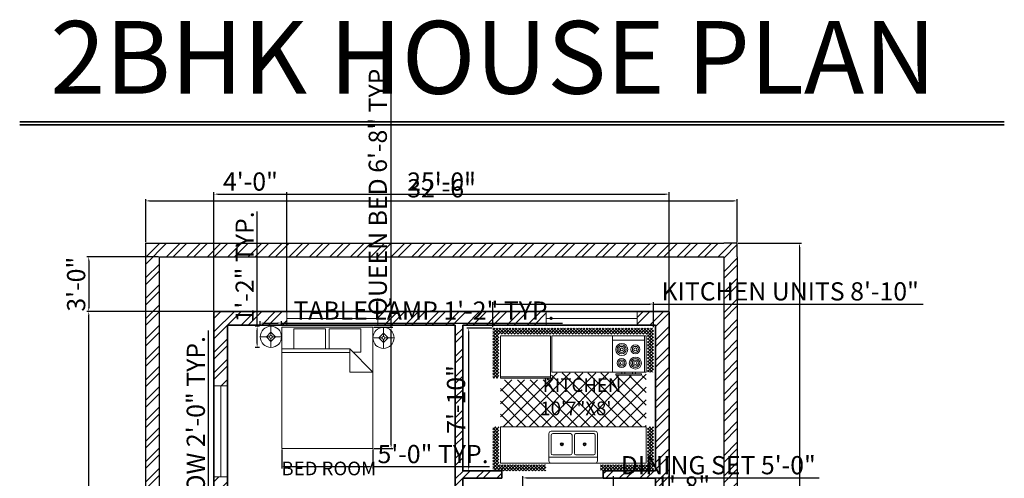
# Model space of a CAD drawing. Units: inches. Extents: x 2588 to 3237, y 2402 to 3178.
# Tile 4 of 4: x 2588 to 3237, y 2876 to 3178. Entities that reach past the tile are written whole.
import ezdxf

# ---------------------------------------------------------------- set-up
doc = ezdxf.new("R2010")
doc.units = ezdxf.units.IN
for name, color, linetype, lineweight in [('A-ANNO-DIMS', 2, 'Continuous', 18), ('A-ANNO-TITL', 7, 'Continuous', 35), ('A-AREA-IDEN', 7, 'Continuous', 25), ('A-FLOR-FIXT', 9, 'Continuous', 18), ('A-FURN', 8, 'Continuous', 18), ('A-GLAZ', 4, 'Continuous', 18), ('A-WALL-PATT', 252, 'Continuous', 13), ('L-WALL', 7, 'Continuous', 30), ('L-WALL-PATT', 252, 'Continuous', 13), ('wall', 210, 'Continuous', 35)]:
    doc.layers.add(name, color=color, linetype=linetype, lineweight=lineweight)
doc.styles.get("Standard").update_dxf_attribs({"font": 'arial.ttf'})
doc.dimstyles.new('ISO-25', dxfattribs={"dimtxt": 12, "dimasz": 2.5, "dimexe": 1.25, "dimexo": 0.625, "dimtad": 1, "dimdec": 1, "dimlunit": 4, "dimtxsty": 'Standard', "dimcen": 2.5, "dimadec": 0, "dimazin": 0, "dimtfac": 1, "dimtdec": 1, "dimtmove": 0, "dimatfit": 3, "dimfxl": 1, "dimarcsym": 0})

# ---------------------------------------------------------------- blocks, each defined once
blk = doc.blocks.new('Kitchen Layout - 7 x 8 ft')
for p, q in [((-5, 81.32), (2.68, 89)), ((-5, 83.44), (0.56, 89)), ((-5, 85.56), (-1.56, 89)), ((-5, 87.68), (-3.68, 89)), ((-1, 84.97), (-5, 88.97)), ((-1, 82.85), (-5, 86.85)), ((-1, 80.73), (-5, 84.73)), ((1.09, 85), (-2.91, 89)), ((3.21, 85), (-0.79, 89)), ((0.81, 85), (4.81, 89)), ((5.34, 85), (1.34, 89)), ((2.93, 85), (6.93, 89)), ((7.46, 85), (3.46, 89)), ((5.05, 85), (9.05, 89)), ((9.58, 85), (5.58, 89)), ((7.17, 85), (11.17, 89)), ((11.7, 85), (7.7, 89)), ((9.29, 85), (13.29, 89)), ((13.82, 85), (9.82, 89)), ((11.41, 85), (15.41, 89)), ((15.94, 85), (11.94, 89)), ((13.53, 85), (17.53, 89)), ((18.06, 85), (14.06, 89)), ((15.65, 85), (19.65, 89)), ((20.18, 85), (16.18, 89)), ((17.78, 85), (21.78, 89)), ((22.31, 85), (18.31, 89)), ((19.9, 85), (23.9, 89)), ((24.43, 85), (20.43, 89)), ((22.02, 85), (26.02, 89)), ((26.55, 85), (22.55, 89)), ((24.14, 85), (28.14, 89)), ((28.67, 85), (24.67, 89)), ((26.26, 85), (30.26, 89)), ((30.79, 85), (26.79, 89)), ((28.38, 85), (32.38, 89)), ((32.91, 85), (28.91, 89)), ((30.5, 85), (34.5, 89)), ((35.03, 85), (31.03, 89)), ((32.63, 85), (36.63, 89)), ((37.16, 85), (33.16, 89)), ((34.75, 85), (38.75, 89)), ((39.28, 85), (35.28, 89)), ((36.87, 85), (40.87, 89)), ((41.4, 85), (37.4, 89)), ((38.99, 85), (42.99, 89)), ((43.52, 85), (39.52, 89)), ((41.11, 85), (45.11, 89)), ((45.64, 85), (41.64, 89)), ((43.23, 85), (47.23, 89)), ((47.76, 85), (43.76, 89)), ((45.35, 85), (49.35, 89)), ((49.88, 85), (45.88, 89)), ((47.47, 85), (51.47, 89)), ((52, 85), (48, 89)), ((49.6, 85), (53.6, 89)), ((54.13, 85), (50.13, 89)), ((51.72, 85), (55.72, 89)), ((56.25, 85), (52.25, 89)), ((53.84, 85), (57.84, 89)), ((58.37, 85), (54.37, 89)), ((55.96, 85), (59.96, 89)), ((60.49, 85), (56.49, 89)), ((58.08, 85), (62.08, 89)), ((62.61, 85), (58.61, 89)), ((60.2, 85), (64.2, 89)), ((64.73, 85), (60.73, 89)), ((62.32, 85), (66.32, 89)), ((66.85, 85), (62.85, 89)), ((64.45, 85), (68.45, 89)), ((68.97, 85), (64.97, 89)), ((66.57, 85), (70.57, 89)), ((71.1, 85), (67.1, 89)), ((68.69, 85), (72.69, 89)), ((73.22, 85), (69.22, 89)), ((70.81, 85), (74.81, 89)), ((75.34, 85), (71.34, 89)), ((72.93, 85), (76.93, 89)), ((77.46, 85), (73.46, 89)), ((75.05, 85), (79.05, 89)), ((79.58, 85), (75.58, 89)), ((77.17, 85), (81.17, 89)), ((81.7, 85), (77.7, 89)), ((79.29, 85), (83.29, 89)), ((83.82, 85), (79.82, 89)), ((81.42, 85), (85.42, 89)), ((85.95, 85), (81.95, 89)), ((83.54, 85), (87.54, 89)), ((88.07, 85), (84.07, 89)), ((85.66, 85), (89.66, 89)), ((90.19, 85), (86.19, 89)), ((87.78, 85), (91.78, 89)), ((92.31, 85), (88.31, 89)), ((89.9, 85), (93.9, 89)), ((94.43, 85), (90.43, 89)), ((92.02, 85), (96.02, 89)), ((96.55, 85), (92.55, 89)), ((94.14, 85), (98.14, 89)), ((101, 82.67), (94.67, 89)), ((96.27, 85), (100.27, 89)), ((101, 84.79), (96.79, 89)), ((97, 83.61), (101, 87.61)), ((97, 81.49), (101, 85.49)), ((101, 80.55), (97, 84.55)), ((101, 86.92), (98.92, 89)), ((-5, 79.19), (-1, 83.19)), ((-1, 78.61), (-5, 82.61)), ((-5, 77.07), (-1, 81.07)), ((-1, 76.49), (-5, 80.49)), ((-5, 74.95), (-1, 78.95)), ((-1, 74.36), (-5, 78.36)), ((34, 84), (96, 84)), ((34, 60), (34, 84)), ((74, 81), (95, 81)), ((96, 84), (96, 60)), ((97, 79.37), (101, 83.37)), ((101, 78.43), (97, 82.43)), ((97, 77.25), (101, 81.25)), ((101, 76.31), (97, 80.31)), ((97, 75.13), (101, 79.13)), ((101, 74.19), (97, 78.19)), ((-5, 72.83), (-1, 76.83)), ((-1, 72.24), (-5, 76.24)), ((-5, 70.71), (-1, 74.71)), ((-1, 70.12), (-5, 74.12)), ((-5, 68.59), (-1, 72.59)), ((-1, 68), (-5, 72)), ((97, 73.01), (101, 77.01)), ((101, 72.07), (97, 76.07)), ((97, 70.89), (101, 74.89)), ((101, 69.95), (97, 73.95)), ((97, 68.76), (101, 72.76)), ((101, 67.82), (97, 71.82)), ((-5, 66.47), (-1, 70.47)), ((-1, 65.88), (-5, 69.88)), ((-5, 64.35), (-1, 68.35)), ((-1, 63.76), (-5, 67.76)), ((-5, 62.22), (-1, 66.22)), ((-1, 61.64), (-5, 65.64)), ((97, 66.64), (101, 70.64)), ((101, 65.7), (97, 69.7)), ((97, 64.52), (101, 68.52)), ((101, 63.58), (97, 67.58)), ((97, 62.4), (101, 66.4)), ((101, 61.46), (97, 65.46)), ((-5, 60.1), (-1, 64.1)), ((-1, 59.52), (-5, 63.52)), ((-5, 57.98), (-1, 61.98)), ((-1, 57.39), (-5, 61.39)), ((-1.73, 56), (-5, 59.27)), ((-4.86, 56), (-1, 59.86)), ((10.4, 24), (45.9, 59.5)), ((18.88, 24), (54.38, 59.5)), ((27.37, 24), (62.87, 59.5)), ((33.03, 55.11), (37.41, 59.5)), ((96, 60), (34, 60)), ((35.85, 24), (71.35, 59.5)), ((76.2, 24), (40.7, 59.5)), ((84.68, 24), (49.18, 59.5)), ((93.17, 24), (57.67, 59.5)), ((61.31, 24), (96, 58.69)), ((96, 29.65), (66.15, 59.5)), ((80, 60), (80, 59)), ((82, 59), (82, 60)), ((87, 59), (87, 60)), ((89, 60), (89, 59)), ((97, 60.28), (101, 64.28)), ((100.34, 60), (97, 63.34)), ((98.22, 60), (97, 61.22)), ((98.84, 60), (101, 62.16)), ((100.96, 60), (101, 60.04)), ((-3.85, 56), (-5, 57.15)), ((-2.74, 56), (-1, 57.74)), ((0, 57), (33, 57)), ((0, 30.57), (24.43, 55)), ((0, 39.06), (15.94, 55)), ((0, 47.54), (7.46, 55)), ((1.91, 24), (32.91, 55)), ((33.77, 24), (2.77, 55)), ((42.26, 24), (11.26, 55)), ((50.74, 24), (19.74, 55)), ((59.23, 24), (28.23, 55)), ((31, 55), (31, 56)), ((32, 55), (31, 55)), ((32, 56), (32, 55)), ((67.71, 24), (33.68, 58.04)), ((44.34, 24), (77.84, 57.5)), ((52.82, 24), (86.32, 57.5)), ((96, 38.14), (76.64, 57.5)), ((96, 46.63), (85.13, 57.5)), ((96, 55.11), (93.57, 57.54)), ((25.29, 24), (0, 49.29)), ((69.79, 24), (96, 50.21)), ((16.8, 24), (0, 40.8)), ((78.28, 24), (96, 41.72)), ((86.76, 24), (96, 33.24)), ((8.32, 24), (0, 32.32)), ((-5, 21.92), (-2.92, 24)), ((-5, 19.8), (-1, 23.8)), ((-1, 19.21), (-5, 23.21)), ((-5, 17.68), (-1, 21.68)), ((-1, 17.09), (-5, 21.09)), ((-5, 15.55), (-1, 19.55)), ((-1, 21.33), (-3.67, 24)), ((-1, 23.45), (-1.55, 24)), ((0, 24), (96, 24)), ((0, 0), (0, 24)), ((95.25, 24), (96, 24.75)), ((96, 24), (96, 0)), ((97, 22.1), (98.9, 24)), ((97, 19.97), (101, 23.97)), ((101, 19.03), (97, 23.03)), ((97, 17.85), (101, 21.85)), ((101, 16.91), (97, 20.91)), ((97, 15.73), (101, 19.73)), ((101, 21.16), (98.16, 24)), ((101, 23.28), (100.28, 24)), ((-1, 14.97), (-5, 18.97)), ((-5, 13.43), (-1, 17.43)), ((-1, 12.85), (-5, 16.85)), ((-5, 11.31), (-1, 15.31)), ((-1, 10.73), (-5, 14.73)), ((-5, 9.19), (-1, 13.19)), ((47.25, 6.5), (47.25, 18.5)), ((48.75, 18.5), (48.75, 6.5)), ((101, 14.79), (97, 18.79)), ((97, 13.61), (101, 17.61)), ((101, 12.67), (97, 16.67)), ((97, 11.49), (101, 15.49)), ((101, 10.55), (97, 14.55)), ((97, 9.37), (101, 13.37)), ((-1, 8.6), (-5, 12.6)), ((-5, 7.07), (-1, 11.07)), ((-1, 6.48), (-5, 10.48)), ((-5, 4.95), (-1, 8.95)), ((-1, 4.36), (-5, 8.36)), ((-5, 2.83), (-1, 6.83)), ((101, 8.43), (97, 12.43)), ((97, 7.25), (101, 11.25)), ((101, 6.31), (97, 10.31)), ((97, 5.12), (101, 9.12)), ((101, 4.18), (97, 8.18)), ((97, 3), (101, 7)), ((-1, 2.24), (-5, 6.24)), ((-5, 0.71), (-1, 4.71)), ((-1, 0.12), (-5, 4.12)), ((-5, -1.42), (-1, 2.58)), ((2, -5), (-5, 2)), ((-5, -3.54), (-1, 0.46)), ((96, 0), (0, 0)), ((64, 4), (32, 4)), ((93.24, -5), (101, 2.76)), ((95.36, -5), (101, 0.64)), ((101, 2.06), (97, 6.06)), ((97, 0.88), (101, 4.88)), ((101, -0.06), (97, 3.94)), ((101, -2.18), (97, 1.82)), ((-0.12, -5), (-5, -0.12)), ((-2.25, -5), (-5, -2.25)), ((-4.37, -5), (-5, -4.37)), ((-4.34, -5), (-0.34, -1)), ((-2.22, -5), (1.78, -1)), ((-0.1, -5), (3.9, -1)), ((4.12, -5), (0.12, -1)), ((2.02, -5), (6.02, -1)), ((6.24, -5), (2.24, -1)), ((4.14, -5), (8.14, -1)), ((8.36, -5), (4.36, -1)), ((6.27, -5), (10.27, -1)), ((10.48, -5), (6.48, -1)), ((8.39, -5), (12.39, -1)), ((12.6, -5), (8.6, -1)), ((10.51, -5), (14.51, -1)), ((14.73, -5), (10.73, -1)), ((12.63, -5), (16.63, -1)), ((16.85, -5), (12.85, -1)), ((14.75, -5), (18.75, -1)), ((18.97, -5), (14.97, -1)), ((16.87, -5), (20.87, -1)), ((21.09, -5), (17.09, -1)), ((18.99, -5), (22.99, -1)), ((23.21, -5), (19.21, -1)), ((21.11, -5), (25.11, -1)), ((25.33, -5), (21.33, -1)), ((23.24, -5), (27.24, -1)), ((27.45, -5), (23.45, -1)), ((25.36, -5), (29.36, -1)), ((29.57, -5), (25.57, -1)), ((27.48, -5), (30, -2.48)), ((30, -3.3), (27.7, -1)), ((29.6, -5), (30, -4.6)), ((30, -1.18), (29.82, -1)), ((66, -2.54), (67.54, -1)), ((66, -4.66), (69.66, -1)), ((69.88, -5), (66, -1.12)), ((67.76, -5), (66, -3.24)), ((67.78, -5), (71.78, -1)), ((72, -5), (68, -1)), ((69.9, -5), (73.9, -1)), ((74.12, -5), (70.12, -1)), ((72.03, -5), (76.03, -1)), ((76.24, -5), (72.24, -1)), ((74.15, -5), (78.15, -1)), ((78.36, -5), (74.36, -1)), ((76.27, -5), (80.27, -1)), ((80.49, -5), (76.49, -1)), ((78.39, -5), (82.39, -1)), ((82.61, -5), (78.61, -1)), ((80.51, -5), (84.51, -1)), ((84.73, -5), (80.73, -1)), ((82.63, -5), (86.63, -1)), ((86.85, -5), (82.85, -1)), ((84.75, -5), (88.75, -1)), ((88.97, -5), (84.97, -1)), ((86.88, -5), (90.88, -1)), ((91.09, -5), (87.09, -1)), ((89, -5), (93, -1)), ((93.21, -5), (89.21, -1)), ((91.12, -5), (95.12, -1)), ((95.34, -5), (91.34, -1)), ((97.46, -5), (93.46, -1)), ((99.58, -5), (95.58, -1)), ((101, -4.3), (97, -0.3)), ((97.48, -5), (101, -1.48)), ((99.6, -5), (101, -3.6))]:
    blk.add_line(p, q)
for points in [[(0, 56), (0, 84), (33, 84), (33, 56)], [(74, 60), (74, 84), (95, 84), (95, 60)], [(76, 58), (76, 59), (93, 59), (93, 58)]]:
    blk.add_lwpolyline(points, close=True)
for points in [[(32, 1.5), (32, 19.5)], [(33.5, 21), (62.5, 21)], [(34.5, 19.5), (46.25, 19.5)], [(49.75, 19.5), (61.5, 19.5)], [(64, 19.5), (64, 1.5)], [(33.5, 6.5), (33.5, 18.5)], [(62.5, 18.5), (62.5, 6.5)], [(62.5, 0), (33.5, 0)], [(46.25, 5.5), (34.5, 5.5)], [(61.5, 5.5), (49.75, 5.5)]]:
    blk.add_lwpolyline(points)
for centre, radius in [((80, 75), 4), ((80, 75), 3), ((89, 75), 3), ((80, 75), 2), ((80, 75), 1), ((89, 75), 2), ((89, 75), 1), ((80, 66), 3), ((80, 66), 2), ((80, 66), 1), ((89, 66), 4), ((89, 66), 3), ((89, 66), 2), ((89, 66), 1), ((40.5, 12.5), 1), ((40.5, 12.5), 0.5), ((55.5, 12.5), 1), ((55.5, 12.5), 0.5)]:
    blk.add_circle(centre, radius)
for centre, radius, start, end in [((33.5, 19.5), 1.5, 90, 180), ((34.5, 18.5), 1, 90, 180), ((46.25, 18.5), 1, 0, 90), ((49.75, 18.5), 1, 90, 180), ((61.5, 18.5), 1, 0, 90), ((62.5, 19.5), 1.5, 0, 90), ((34.5, 6.5), 1, 180, 270), ((46.25, 6.5), 1, 270, 0), ((49.75, 6.5), 1, 180, 270), ((61.5, 6.5), 1, 270, 0), ((33.5, 1.5), 1.5, 180, 270), ((62.5, 1.5), 1.5, 270, 0)]:
    blk.add_arc(centre, radius, start, end)
blk = doc.blocks.new('Bed - Queen')
for p, q in [((0, -80.00003), (0, 0)), ((0, 0), (59.99999, 0)), ((59.99999, 0), (59.99999, -80.00003)), ((7.99999, -1.2), (28.79998, -1.2)), ((7.99999, -14.4), (7.99999, -1.2)), ((28.79998, -1.2), (28.79998, -14.4)), ((31.19999, -1.2), (51.99999, -1.2)), ((31.19999, -14.4), (31.19999, -1.2)), ((51.99999, -1.2), (51.99999, -16.4)), ((0, -14.4), (44.8, -14.4)), ((44.8, -16.8), (0, -16.8)), ((59.99999, -29.6), (44.8, -14.4)), ((44.8, -14.4), (44.8, -29.6)), ((51.99999, -16.4), (46.79936, -16.4)), ((44.8, -29.6), (59.99999, -29.6)), ((59.99999, -80.00003), (0, -80.00003))]:
    blk.add_line(p, q)
blk = doc.blocks.new('Lamp - Table')
for p, q in [((0, 7), (0, 1)), ((-1, 0), (-7, 0)), ((0, 3), (-3, 0)), ((-3, 0), (0, -3)), ((3, 0), (0, 3)), ((0, -3), (3, 0)), ((1, 0), (7, 0)), ((0, -1), (0, -7))]:
    blk.add_line(p, q)
for radius in [7, 1]:
    blk.add_circle((0, 0), radius)
blk = doc.blocks.new('*D22')
at = {"layer": 'A-ANNO-DIMS', "color": 0, "lineweight": -2, "transparency": 16777216}
for p, q in [((2671.4, 3031.46), (2671.4, 3060.02)), ((2673.9, 3058.77), (3058.9, 3058.77)), ((3061.4, 3031.46), (3061.4, 3060.02))]:
    blk.add_line(p, q, dxfattribs=at)
at = {"layer": 'A-ANNO-DIMS', "color": 0, "transparency": 16777216}
for points in [[(2673.9, 3059.19), (2673.9, 3058.36), (2671.4, 3058.77)], [(3058.9, 3059.19), (3058.9, 3058.36), (3061.4, 3058.77)]]:
    blk.add_solid(points, dxfattribs=at)
at = {"layer": 'Defpoints', "color": 0, "transparency": 16777216}
for p in [(3061.4, 3058.77), (2671.4, 3030.83), (3061.4, 3030.83)]:
    blk.add_point(p, dxfattribs=at)
at = {"layer": 'A-ANNO-DIMS', "color": 0, "transparency": 16777216, "insert": (2866.4, 3065.53), "char_height": 12, "attachment_point": 5}
blk.add_mtext('32\'-6"', dxfattribs=at)
blk = doc.blocks.new('*D23')
at = {"layer": 'A-ANNO-DIMS', "color": 0, "lineweight": -2, "transparency": 16777216}
for p, q in [((3062.02, 3030.83), (3103.65, 3030.83)), ((3102.4, 3028.33), (3102.4, 2475.33)), ((3062.02, 2472.83), (3103.65, 2472.83))]:
    blk.add_line(p, q, dxfattribs=at)
at = {"layer": 'A-ANNO-DIMS', "color": 0, "transparency": 16777216}
for points in [[(3101.99, 3028.33), (3102.82, 3028.33), (3102.4, 3030.83)], [(3101.99, 2475.33), (3102.82, 2475.33), (3102.4, 2472.83)]]:
    blk.add_solid(points, dxfattribs=at)
at = {"layer": 'Defpoints', "color": 0, "transparency": 16777216}
for p in [(3061.4, 3030.83), (3061.4, 2472.83), (3102.4, 2472.83)]:
    blk.add_point(p, dxfattribs=at)
at = {"layer": 'A-ANNO-DIMS', "color": 0, "transparency": 16777216, "insert": (3095.65, 2751.83), "char_height": 12, "attachment_point": 5, "rotation": 90}
blk.add_mtext('46\'-6"', dxfattribs=at)
blk = doc.blocks.new('WIN-60IN')
blk.add_line((4.5, 60), (4.5, 0))
blk.add_lwpolyline([(9, 60), (9, 0), (0, 0), (0, 60)], close=True)
blk = doc.blocks.new('*D28')
at = {"layer": 'A-ANNO-DIMS', "color": 0, "lineweight": -2, "transparency": 16777216}
for p, q in [((2833.13, 2975.52), (2833.13, 3155.79)), ((2821.75, 2975.52), (2834.38, 2975.52)), ((2833.13, 2898.02), (2833.13, 2973.02)), ((2821.75, 2895.52), (2834.38, 2895.52))]:
    blk.add_line(p, q, dxfattribs=at)
at = {"layer": 'A-ANNO-DIMS', "color": 0, "transparency": 16777216}
for points in [[(2832.71, 2973.02), (2833.55, 2973.02), (2833.13, 2975.52)], [(2832.71, 2898.02), (2833.55, 2898.02), (2833.13, 2895.52)]]:
    blk.add_solid(points, dxfattribs=at)
at = {"layer": 'Defpoints', "color": 0, "transparency": 16777216}
for p in [(2821.13, 2975.52), (2833.13, 2975.52), (2821.13, 2895.52)]:
    blk.add_point(p, dxfattribs=at)
at = {"layer": 'A-ANNO-DIMS', "color": 0, "transparency": 16777216, "insert": (2825.93, 3066.9), "char_height": 12, "attachment_point": 5, "rotation": 90}
blk.add_mtext('QUEEN BED 6\'-8" TYP.', dxfattribs=at)
blk = doc.blocks.new('*D29')
at = {"layer": 'A-ANNO-DIMS', "color": 0, "lineweight": -2, "transparency": 16777216}
for p, q in [((2761.13, 2894.89), (2761.13, 2882.27)), ((2821.13, 2894.89), (2821.13, 2882.27)), ((2763.63, 2883.52), (2818.63, 2883.52)), ((2821.13, 2883.52), (2898.03, 2883.52))]:
    blk.add_line(p, q, dxfattribs=at)
at = {"layer": 'A-ANNO-DIMS', "color": 0, "transparency": 16777216}
for points in [[(2763.63, 2883.93), (2763.63, 2883.1), (2761.13, 2883.52)], [(2818.63, 2883.93), (2818.63, 2883.1), (2821.13, 2883.52)]]:
    blk.add_solid(points, dxfattribs=at)
at = {"layer": 'Defpoints', "color": 0, "transparency": 16777216}
for p in [(2761.13, 2895.52), (2821.13, 2895.52), (2821.13, 2883.52)]:
    blk.add_point(p, dxfattribs=at)
at = {"layer": 'A-ANNO-DIMS', "color": 0, "transparency": 16777216, "insert": (2860.83, 2890.27), "char_height": 12, "attachment_point": 5}
blk.add_mtext('5\'-0" TYP.', dxfattribs=at)
blk = doc.blocks.new('*D30')
at = {"layer": 'A-ANNO-DIMS', "color": 0, "lineweight": -2, "transparency": 16777216}
for p, q in [((2746.93, 2976.75), (2746.93, 2979.48)), ((2760.93, 2976.75), (2760.93, 2979.48)), ((2749.43, 2978.23), (2758.43, 2978.23)), ((2760.93, 2978.23), (2946.2, 2978.23))]:
    blk.add_line(p, q, dxfattribs=at)
at = {"layer": 'A-ANNO-DIMS', "color": 0, "transparency": 16777216}
for points in [[(2749.43, 2978.64), (2749.43, 2977.81), (2746.93, 2978.23)], [(2758.43, 2978.64), (2758.43, 2977.81), (2760.93, 2978.23)]]:
    blk.add_solid(points, dxfattribs=at)
at = {"layer": 'Defpoints', "color": 0, "transparency": 16777216}
for p in [(2746.93, 2976.13), (2760.93, 2978.23), (2760.93, 2976.13)]:
    blk.add_point(p, dxfattribs=at)
at = {"layer": 'A-ANNO-DIMS', "color": 0, "transparency": 16777216, "insert": (2854.82, 2984.88), "char_height": 12, "attachment_point": 5}
blk.add_mtext('TABLE LAMP 1\'-2" TYP.', dxfattribs=at)
blk = doc.blocks.new('*D31')
at = {"layer": 'A-ANNO-DIMS', "color": 0, "lineweight": -2, "transparency": 16777216}
for p, q in [((2744.83, 2976.13), (2744.83, 3051.89)), ((2746.31, 2976.13), (2743.58, 2976.13)), ((2744.83, 2964.63), (2744.83, 2973.63)), ((2746.31, 2962.13), (2743.58, 2962.13))]:
    blk.add_line(p, q, dxfattribs=at)
at = {"layer": 'A-ANNO-DIMS', "color": 0, "transparency": 16777216}
for points in [[(2744.41, 2973.63), (2745.25, 2973.63), (2744.83, 2976.13)], [(2744.41, 2964.63), (2745.25, 2964.63), (2744.83, 2962.13)]]:
    blk.add_solid(points, dxfattribs=at)
at = {"layer": 'Defpoints', "color": 0, "transparency": 16777216}
for p in [(2744.83, 2976.13), (2746.93, 2976.13), (2746.93, 2962.13)]:
    blk.add_point(p, dxfattribs=at)
at = {"layer": 'A-ANNO-DIMS', "color": 0, "transparency": 16777216, "insert": (2738.18, 3015.26), "char_height": 12, "attachment_point": 5, "rotation": 90}
blk.add_mtext('1\'-2" TYP.', dxfattribs=at)
blk = doc.blocks.new('*D32')
at = {"layer": 'A-ANNO-DIMS', "color": 0, "lineweight": -2, "transparency": 16777216}
for p, q in [((2712.8, 2817.75), (2712.8, 2973.35)), ((2715.77, 2817.75), (2711.55, 2817.75)), ((2712.8, 2796.25), (2712.8, 2815.25)), ((2715.77, 2793.75), (2711.55, 2793.75))]:
    blk.add_line(p, q, dxfattribs=at)
at = {"layer": 'A-ANNO-DIMS', "color": 0, "transparency": 16777216}
for points in [[(2712.38, 2815.25), (2713.21, 2815.25), (2712.8, 2817.75)], [(2712.38, 2796.25), (2713.21, 2796.25), (2712.8, 2793.75)]]:
    blk.add_solid(points, dxfattribs=at)
at = {"layer": 'Defpoints', "color": 0, "transparency": 16777216}
for p in [(2712.8, 2817.75), (2716.4, 2817.75), (2716.4, 2793.75)]:
    blk.add_point(p, dxfattribs=at)
at = {"layer": 'A-ANNO-DIMS', "color": 0, "transparency": 16777216, "insert": (2705.96, 2896.8), "char_height": 12, "attachment_point": 5, "rotation": 90}
blk.add_mtext('WINDOW 2\'-0" TYP.', dxfattribs=at)
blk = doc.blocks.new('*D34')
at = {"layer": 'A-ANNO-DIMS', "color": 0, "lineweight": -2, "transparency": 16777216}
for p, q in [((2900.2, 2975.46), (2900.2, 2991.98)), ((2902.7, 2990.73), (3003.7, 2990.73)), ((3006.2, 2975.46), (3006.2, 2991.98)), ((3006.2, 2990.73), (3183.83, 2990.73))]:
    blk.add_line(p, q, dxfattribs=at)
at = {"layer": 'A-ANNO-DIMS', "color": 0, "transparency": 16777216}
for points in [[(2902.7, 2991.15), (2902.7, 2990.32), (2900.2, 2990.73)], [(3003.7, 2991.15), (3003.7, 2990.32), (3006.2, 2990.73)]]:
    blk.add_solid(points, dxfattribs=at)
at = {"layer": 'Defpoints', "color": 0, "transparency": 16777216}
for p in [(3006.2, 2990.73), (2900.2, 2974.83), (3006.2, 2974.83)]:
    blk.add_point(p, dxfattribs=at)
at = {"layer": 'A-ANNO-DIMS', "color": 0, "transparency": 16777216, "insert": (3096.26, 2997.56), "char_height": 12, "attachment_point": 5}
blk.add_mtext('KITCHEN UNITS 8\'-10"', dxfattribs=at)
blk = doc.blocks.new('*D35')
at = {"layer": 'A-ANNO-DIMS', "color": 0, "lineweight": -2, "transparency": 16777216}
for p, q in [((2899.57, 2974.83), (2883.05, 2974.83)), ((2884.3, 2883.33), (2884.3, 2972.33)), ((2899.57, 2880.83), (2883.05, 2880.83))]:
    blk.add_line(p, q, dxfattribs=at)
at = {"layer": 'A-ANNO-DIMS', "color": 0, "transparency": 16777216}
for points in [[(2883.88, 2972.33), (2884.72, 2972.33), (2884.3, 2974.83)], [(2883.88, 2883.33), (2884.72, 2883.33), (2884.3, 2880.83)]]:
    blk.add_solid(points, dxfattribs=at)
at = {"layer": 'Defpoints', "color": 0, "transparency": 16777216}
for p in [(2884.3, 2974.83), (2900.2, 2974.83), (2900.2, 2880.83)]:
    blk.add_point(p, dxfattribs=at)
at = {"layer": 'A-ANNO-DIMS', "color": 0, "transparency": 16777216, "insert": (2877.55, 2927.83), "char_height": 12, "attachment_point": 5, "rotation": 90}
blk.add_mtext('7\'-10"', dxfattribs=at)
blk = doc.blocks.new('*D36')
at = {"layer": 'A-ANNO-DIMS', "color": 0, "lineweight": -2, "transparency": 16777216}
for p, q in [((2919.92, 2867.74), (2919.92, 2877.35)), ((2922.42, 2876.1), (2977.29, 2876.1)), ((2979.79, 2867.74), (2979.79, 2877.35)), ((2979.79, 2876.1), (3115.43, 2876.1))]:
    blk.add_line(p, q, dxfattribs=at)
at = {"layer": 'A-ANNO-DIMS', "color": 0, "transparency": 16777216}
for points in [[(2922.42, 2876.51), (2922.42, 2875.68), (2919.92, 2876.1)], [(2977.29, 2876.51), (2977.29, 2875.68), (2979.79, 2876.1)]]:
    blk.add_solid(points, dxfattribs=at)
at = {"layer": 'Defpoints', "color": 0, "transparency": 16777216}
for p in [(2979.79, 2876.1), (2919.92, 2867.12), (2979.79, 2867.12)]:
    blk.add_point(p, dxfattribs=at)
at = {"layer": 'A-ANNO-DIMS', "color": 0, "transparency": 16777216, "insert": (3048.86, 2882.93), "char_height": 12, "attachment_point": 5}
blk.add_mtext('DINING SET 5\'-0"', dxfattribs=at)
blk = doc.blocks.new('*D39')
at = {"layer": 'A-ANNO-DIMS', "color": 0, "lineweight": -2, "transparency": 16777216}
for p, q in [((2986.73, 2859.73), (2986.73, 2864.04)), ((2989.23, 2862.79), (3004.37, 2862.79)), ((3006.87, 2859.73), (3006.87, 2864.04)), ((3006.87, 2862.79), (3041.39, 2862.79))]:
    blk.add_line(p, q, dxfattribs=at)
at = {"layer": 'A-ANNO-DIMS', "color": 0, "transparency": 16777216}
for points in [[(2989.23, 2863.21), (2989.23, 2862.37), (2986.73, 2862.79)], [(3004.37, 2863.21), (3004.37, 2862.37), (3006.87, 2862.79)]]:
    blk.add_solid(points, dxfattribs=at)
at = {"layer": 'Defpoints', "color": 0, "transparency": 16777216}
for p in [(3006.87, 2862.79), (2986.73, 2859.11), (3006.87, 2859.11)]:
    blk.add_point(p, dxfattribs=at)
at = {"layer": 'A-ANNO-DIMS', "color": 0, "transparency": 16777216, "insert": (3025.38, 2869.54), "char_height": 12, "attachment_point": 5}
blk.add_mtext('1\'-8"', dxfattribs=at)
blk = doc.blocks.new('*D46')
at = {"layer": 'A-ANNO-DIMS', "color": 0, "lineweight": -2, "transparency": 16777216}
for p, q in [((2716.4, 2986.46), (2716.4, 3064.48)), ((2764.42, 2986.46), (2764.42, 3064.48)), ((2718.9, 3063.23), (2761.92, 3063.23))]:
    blk.add_line(p, q, dxfattribs=at)
at = {"layer": 'A-ANNO-DIMS', "color": 0, "transparency": 16777216}
for points in [[(2718.9, 3063.65), (2718.9, 3062.82), (2716.4, 3063.23)], [(2761.92, 3063.65), (2761.92, 3062.82), (2764.42, 3063.23)]]:
    blk.add_solid(points, dxfattribs=at)
at = {"layer": 'Defpoints', "color": 0, "transparency": 16777216}
for p in [(2764.42, 3063.23), (2716.4, 2985.83), (2764.42, 2985.83)]:
    blk.add_point(p, dxfattribs=at)
at = {"layer": 'A-ANNO-DIMS', "color": 0, "transparency": 16777216, "insert": (2740.41, 3069.98), "char_height": 12, "attachment_point": 5}
blk.add_mtext('4\'-0"', dxfattribs=at)
blk = doc.blocks.new('*D47')
at = {"layer": 'A-ANNO-DIMS', "color": 0, "lineweight": -2, "transparency": 16777216}
for p, q in [((2716.4, 2986.46), (2716.4, 3064.48)), ((3016.4, 2986.46), (3016.4, 3064.48)), ((2718.9, 3063.23), (3013.9, 3063.23))]:
    blk.add_line(p, q, dxfattribs=at)
at = {"layer": 'A-ANNO-DIMS', "color": 0, "transparency": 16777216}
for points in [[(2718.9, 3063.65), (2718.9, 3062.82), (2716.4, 3063.23)], [(3013.9, 3063.65), (3013.9, 3062.82), (3016.4, 3063.23)]]:
    blk.add_solid(points, dxfattribs=at)
at = {"layer": 'Defpoints', "color": 0, "transparency": 16777216}
for p in [(3016.4, 3063.23), (2716.4, 2985.83), (3016.4, 2985.83)]:
    blk.add_point(p, dxfattribs=at)
at = {"layer": 'A-ANNO-DIMS', "color": 0, "transparency": 16777216, "insert": (2866.4, 3069.98), "char_height": 12, "attachment_point": 5}
blk.add_mtext('25\'-0"', dxfattribs=at)
blk = doc.blocks.new('*D49')
at = {"layer": 'A-ANNO-DIMS', "color": 0, "lineweight": -2, "transparency": 16777216}
for p, q in [((2715.77, 2985.83), (2632.58, 2985.83)), ((2633.83, 2628.33), (2633.83, 2983.33)), ((2715.77, 2625.83), (2632.58, 2625.83))]:
    blk.add_line(p, q, dxfattribs=at)
at = {"layer": 'A-ANNO-DIMS', "color": 0, "transparency": 16777216}
for points in [[(2633.42, 2983.33), (2634.25, 2983.33), (2633.83, 2985.83)], [(2633.42, 2628.33), (2634.25, 2628.33), (2633.83, 2625.83)]]:
    blk.add_solid(points, dxfattribs=at)
at = {"layer": 'Defpoints', "color": 0, "transparency": 16777216}
for p in [(2633.83, 2985.83), (2716.4, 2985.83), (2716.4, 2625.83)]:
    blk.add_point(p, dxfattribs=at)
at = {"layer": 'A-ANNO-DIMS', "color": 0, "transparency": 16777216, "insert": (2627.08, 2805.83), "char_height": 12, "attachment_point": 5, "rotation": 90}
blk.add_mtext('30\'-0"', dxfattribs=at)
blk = doc.blocks.new('*D50')
at = {"layer": 'A-ANNO-DIMS', "color": 0, "lineweight": -2, "transparency": 16777216}
for p, q in [((2679.77, 3021.83), (2632.58, 3021.83)), ((2633.83, 3019.33), (2633.83, 2988.33)), ((2715.77, 2985.83), (2632.58, 2985.83))]:
    blk.add_line(p, q, dxfattribs=at)
at = {"layer": 'A-ANNO-DIMS', "color": 0, "transparency": 16777216}
for points in [[(2633.42, 3019.33), (2634.25, 3019.33), (2633.83, 3021.83)], [(2633.42, 2988.33), (2634.25, 2988.33), (2633.83, 2985.83)]]:
    blk.add_solid(points, dxfattribs=at)
at = {"layer": 'Defpoints', "color": 0, "transparency": 16777216}
for p in [(2680.4, 3021.83), (2633.83, 2985.83), (2716.4, 2985.83)]:
    blk.add_point(p, dxfattribs=at)
at = {"layer": 'A-ANNO-DIMS', "color": 0, "transparency": 16777216, "insert": (2627.08, 3003.83), "char_height": 12, "attachment_point": 5, "rotation": 90}
blk.add_mtext('3\'-0"', dxfattribs=at)

msp = doc.modelspace()

# ---------------------------------------------------------------- hatches: boundary and pattern name
at = {"layer": 'A-WALL-PATT'}
h = msp.add_hatch(dxfattribs=at)
h.set_pattern_fill('ANSI32', color=256)
h.paths.add_polyline_path([(3016.4, 2985.83), (2995.46, 2985.83), (2995.46, 2976.83), (3007.4, 2976.83), (3007.4, 2880.83), (2973.06, 2880.83), (2973.06, 2875.83), (3007.4, 2875.83), (3007.4, 2760.26), (3016.4, 2760.26)])
h.paths.add_polyline_path([(2899.05, 2630.33, -0.03766), (2899.39, 2634.83), (2880.4, 2634.83), (2880.4, 2773.83), (2865, 2773.83), (2865, 2769.59, -0.00634), (2864.99, 2768.83), (2875.4, 2768.83), (2875.4, 2634.83), (2836.4, 2634.83), (2836.4, 2625.83), (2899.05, 2625.83)])
h.paths.add_polyline_path([(2725.4, 2734.72), (2716.4, 2734.72), (2716.4, 2702.67), (2725.4, 2702.67)])
h.paths.add_polyline_path([(2776.4, 2634.83), (2725.4, 2634.83), (2725.4, 2642.67), (2716.4, 2642.67), (2716.4, 2625.83), (2776.4, 2625.83)])
h.paths.add_polyline_path([(2725.4, 2793.75), (2716.4, 2793.75), (2716.4, 2758.72), (2725.4, 2758.72), (2725.4, 2768.83), (2815.4, 2768.83), (2815.4, 2752.5), (2816.2, 2752.5), (2820.4, 2752.5), (2820.4, 2768.83), (2835, 2768.83), (2835, 2769.59), (2835, 2773.83), (2820.4, 2773.83), (2820.4, 2785.18), (2816.11, 2785.18, -0.005966), (2815.4, 2785.19), (2815.4, 2773.83), (2725.4, 2773.83)])
h.paths.add_polyline_path([(2725.4, 2876.72), (2716.4, 2876.72), (2716.4, 2817.75), (2725.4, 2817.75), (2725.4, 2827.83), (2815.4, 2827.83), (2815.4, 2815.18), (2816.11, 2815.18), (2820.4, 2815.18), (2820.4, 2827.83), (2836.34, 2827.83), (2836.34, 2832.33), (2836.34, 2832.83), (2725.4, 2832.83)])
h.paths.add_polyline_path([(2725.4, 2976.83), (2764.42, 2976.83), (2764.42, 2985.83), (2716.4, 2985.83), (2716.4, 2936.72), (2725.4, 2936.72)])
h.paths.add_polyline_path([(2935.46, 2985.83), (2824.42, 2985.83), (2824.42, 2976.83), (2875.4, 2976.83), (2875.4, 2832.83), (2866.34, 2832.83, -0.004167), (2866.34, 2832.33), (2866.34, 2827.83), (2880.4, 2827.83), (2880.4, 2875.83), (2906.11, 2875.83), (2906.11, 2880.83), (2880.4, 2880.83), (2880.4, 2976.83), (2935.46, 2976.83)])
at = {"layer": 'L-WALL-PATT'}
h = msp.add_hatch(dxfattribs=at)
h.set_pattern_fill('ANSI32', color=256)
h.paths.add_polyline_path([(3016.4, 2700.26), (3007.4, 2700.26), (3007.4, 2634.83), (2956.08, 2634.83, -0.03766), (2956.42, 2630.33), (2956.42, 2625.83), (3016.4, 2625.83)], flags=17)
h.paths.add_polyline_path([(3061.4, 2985.83), (3061.4, 3021.83), (3061.4, 3030.83), (3052.4, 3030.83), (3016.4, 3030.83), (2716.4, 3030.83), (2680.4, 3030.83), (2671.4, 3030.83), (2671.4, 3021.83), (2671.4, 2985.83), (2671.4, 2625.83), (2671.4, 2481.83), (2671.4, 2472.83), (2680.4, 2472.83), (2716.4, 2472.83), (2836.4, 2472.83), (2900.91, 2472.83), (2900.91, 2481.83), (2836.4, 2481.83), (2716.4, 2481.83), (2680.4, 2481.83), (2680.4, 2625.83), (2680.4, 2985.83), (2680.4, 3021.83), (2716.4, 3021.83), (3016.4, 3021.83), (3052.4, 3021.83), (3052.4, 2985.83), (3052.4, 2625.83), (3052.4, 2481.83), (2984.91, 2481.83), (2984.91, 2472.83), (3052.4, 2472.83), (3061.4, 2472.83), (3061.4, 2481.83), (3061.4, 2625.83)])

# ---------------------------------------------------------------- linework, layer by layer
at = {"layer": 'A-ANNO-TITL'}
for p, q in [((2588.31, 3111.02), (3237.4, 3111.02)), ((2588.31, 3109.02), (3237.4, 3109.02))]:
    msp.add_line(p, q, dxfattribs=at)
at = {"layer": 'L-WALL'}
for p, q in [((2671.4, 3021.83), (2671.4, 3030.83)), ((2671.4, 3030.83), (2680.4, 3030.83)), ((2680.4, 3030.83), (2716.4, 3030.83)), ((2716.4, 3030.83), (3016.4, 3030.83)), ((3016.4, 3030.83), (3052.4, 3030.83)), ((3061.4, 3030.83), (3052.4, 3030.83)), ((3061.4, 3021.83), (3061.4, 3030.83)), ((2671.4, 2985.83), (2671.4, 3021.83)), ((2680.4, 2985.83), (2680.4, 3021.83)), ((2680.4, 3021.83), (2716.4, 3021.83)), ((2716.4, 3021.83), (3016.4, 3021.83)), ((3016.4, 3021.83), (3052.4, 3021.83)), ((3052.4, 3021.83), (3052.4, 2985.83)), ((3061.4, 3021.83), (3061.4, 2985.83)), ((2671.4, 2625.83), (2671.4, 2985.83)), ((2680.4, 2625.83), (2680.4, 2985.83)), ((3052.4, 2985.83), (3052.4, 2625.83)), ((3061.4, 2985.83), (3061.4, 2625.83))]:
    msp.add_line(p, q, dxfattribs=at)
at = {"layer": 'wall'}
for p, q in [((2716.4, 2985.83), (3016.4, 2985.83)), ((2716.4, 2625.83), (2716.4, 2985.83)), ((3016.4, 2985.83), (3016.4, 2625.83)), ((2725.4, 2976.83), (2875.4, 2976.83)), ((2725.4, 2832.83), (2725.4, 2976.83)), ((2875.4, 2832.83), (2875.4, 2976.83)), ((2880.4, 2976.83), (3007.4, 2976.83)), ((2880.4, 2880.83), (2880.4, 2976.83)), ((3007.4, 2976.83), (3007.4, 2880.83)), ((2880.4, 2880.83), (2906.11, 2880.83)), ((2880.4, 2827.83), (2880.4, 2875.83)), ((2880.4, 2875.83), (2906.11, 2875.83)), ((2906.11, 2880.83), (2906.11, 2875.83)), ((2973.06, 2880.83), (2973.06, 2875.83)), ((2973.06, 2880.83), (3007.4, 2880.83)), ((2973.06, 2875.83), (3007.4, 2875.83)), ((3007.4, 2875.83), (3007.4, 2815.83))]:
    msp.add_line(p, q, dxfattribs=at)

# ---------------------------------------------------------------- block references
at = {"layer": 'A-FLOR-FIXT'}
msp.add_blockref('Kitchen Layout - 7 x 8 ft', (2905.2, 2885.83), dxfattribs=at)
at = {"layer": 'A-FURN'}
for name, p in [('Lamp - Table', (2753.93, 2969.13)), ('Bed - Queen', (2761.13, 2975.52)), ('Lamp - Table', (2828.13, 2968.46))]:
    msp.add_blockref(name, p, dxfattribs=at)
at = {"layer": 'A-GLAZ', "rotation": 89.9999999999984}
for p in [(2824.42, 2976.83), (2995.46, 2976.83)]:
    msp.add_blockref('WIN-60IN', p, dxfattribs=at)
at = {"layer": 'A-GLAZ'}
msp.add_blockref('WIN-60IN', (2716.4, 2876.72), dxfattribs=at)

# ---------------------------------------------------------------- texts
at = {"layer": 'A-ANNO-TITL'}
msp.add_text('2BHK HOUSE PLAN', height=48, dxfattribs=at).set_placement((2608.51, 3129.42))
at = {"layer": 'A-AREA-IDEN'}
for s, p in [('KITCHEN', (2933.15, 2932.78)), ('10\'7"X8\'', (2931.53, 2917.43)), ('BED ROOM', (2760.85, 2877.83))]:
    msp.add_text(s, height=9, dxfattribs=at).set_placement(p)

# ---------------------------------------------------------------- dimensions: what is measured, and where the dimension line sits
at = {"layer": 'A-ANNO-DIMS'}
for base, p1, p2, text, picture, middle in [((2833.13, 2975.52), (2821.13, 2895.52), (2821.13, 2975.52), 'QUEEN BED <> TYP.', '*D28', (2825.93, 3066.9)), ((2744.83, 2976.13), (2746.93, 2962.13), (2746.93, 2976.13), '<> TYP.', '*D31', (2738.18, 3015.26)), ((2712.8, 2817.75), (2716.4, 2793.75), (2716.4, 2817.75), 'WINDOW <> TYP.', '*D32', (2705.96, 2896.8))]:
    dim = msp.add_linear_dim(base=base, p1=p1, p2=p2, angle=90, text=text, dimstyle='ISO-25', override={"dimdec": 1, "dimlfac": 1, "dimrnd": 0, "dimzin": 1, "dimdsep": 46, "dimlunit": 4, "dimfrac": 2}, dxfattribs=at)
    dim.commit()
    dim.dimension.update_dxf_attribs({"geometry": picture, "text_midpoint": middle})
for base, p1, p2, override, picture, middle in [((2764.42, 3063.23), (2716.4, 2985.83), (2764.42, 2985.83), {"dimdec": 1, "dimlfac": 1, "dimrnd": 0, "dimzin": 1, "dimdsep": 46, "dimlunit": 4, "dimfrac": 2}, '*D46', (2740.41, 3069.98)), ((3016.4, 3063.23), (2716.4, 2985.83), (3016.4, 2985.83), {"dimdec": 1, "dimlfac": 1, "dimrnd": 0, "dimzin": 1, "dimdsep": 46, "dimlunit": 4, "dimfrac": 2}, '*D47', (2866.4, 3069.98)), ((3061.4, 3058.77), (2671.4, 3030.83), (3061.4, 3030.83), {"dimclrd": 0, "dimclre": 0, "dimclrt": 0}, '*D22', (2866.4, 3065.53)), ((3006.87, 2862.79), (2986.73, 2859.11), (3006.87, 2859.11), {"dimdec": 1, "dimlfac": 1, "dimrnd": 0, "dimzin": 1, "dimdsep": 46, "dimlunit": 4, "dimfrac": 2}, '*D39', (3025.38, 2869.54))]:
    dim = msp.add_linear_dim(base=base, p1=p1, p2=p2, dimstyle='ISO-25', override=override, dxfattribs=at)
    dim.commit()
    dim.dimension.update_dxf_attribs({"geometry": picture, "text_midpoint": middle})
for base, p1, p2, text, picture, middle in [((3006.2, 2990.73), (2900.2, 2974.83), (3006.2, 2974.83), 'KITCHEN UNITS <>', '*D34', (3096.26, 2997.56)), ((2760.93, 2978.23), (2746.93, 2976.13), (2760.93, 2976.13), 'TABLE LAMP <> TYP.', '*D30', (2854.82, 2984.88)), ((2821.13, 2883.52), (2761.13, 2895.52), (2821.13, 2895.52), '<> TYP.', '*D29', (2860.83, 2890.27)), ((2979.79, 2876.1), (2919.92, 2867.12), (2979.79, 2867.12), 'DINING SET <>', '*D36', (3048.86, 2882.93))]:
    dim = msp.add_linear_dim(base=base, p1=p1, p2=p2, text=text, dimstyle='ISO-25', override={"dimdec": 1, "dimlfac": 1, "dimrnd": 0, "dimzin": 1, "dimdsep": 46, "dimlunit": 4, "dimfrac": 2}, dxfattribs=at)
    dim.commit()
    dim.dimension.update_dxf_attribs({"geometry": picture, "text_midpoint": middle})
for base, p1, p2, override, picture, middle in [((3102.4, 2472.83), (3061.4, 3030.83), (3061.4, 2472.83), {"dimclrd": 0, "dimclre": 0, "dimclrt": 0}, '*D23', (3095.65, 2751.83)), ((2633.83, 2985.83), (2680.4, 3021.83), (2716.4, 2985.83), {"dimdec": 1, "dimlfac": 1, "dimrnd": 0, "dimzin": 1, "dimdsep": 46, "dimlunit": 4, "dimfrac": 2}, '*D50', (2627.08, 3003.83)), ((2633.83, 2985.83), (2716.4, 2625.83), (2716.4, 2985.83), {"dimdec": 1, "dimlfac": 1, "dimrnd": 0, "dimzin": 1, "dimdsep": 46, "dimlunit": 4, "dimfrac": 2}, '*D49', (2627.08, 2805.83)), ((2884.3, 2974.83), (2900.2, 2880.83), (2900.2, 2974.83), {"dimdec": 1, "dimlfac": 1, "dimrnd": 0, "dimzin": 1, "dimdsep": 46, "dimlunit": 4, "dimfrac": 2}, '*D35', (2877.55, 2927.83))]:
    dim = msp.add_linear_dim(base=base, p1=p1, p2=p2, angle=90, dimstyle='ISO-25', override=override, dxfattribs=at)
    dim.commit()
    dim.dimension.update_dxf_attribs({"geometry": picture, "text_midpoint": middle})

doc.saveas('drawing.dxf')
